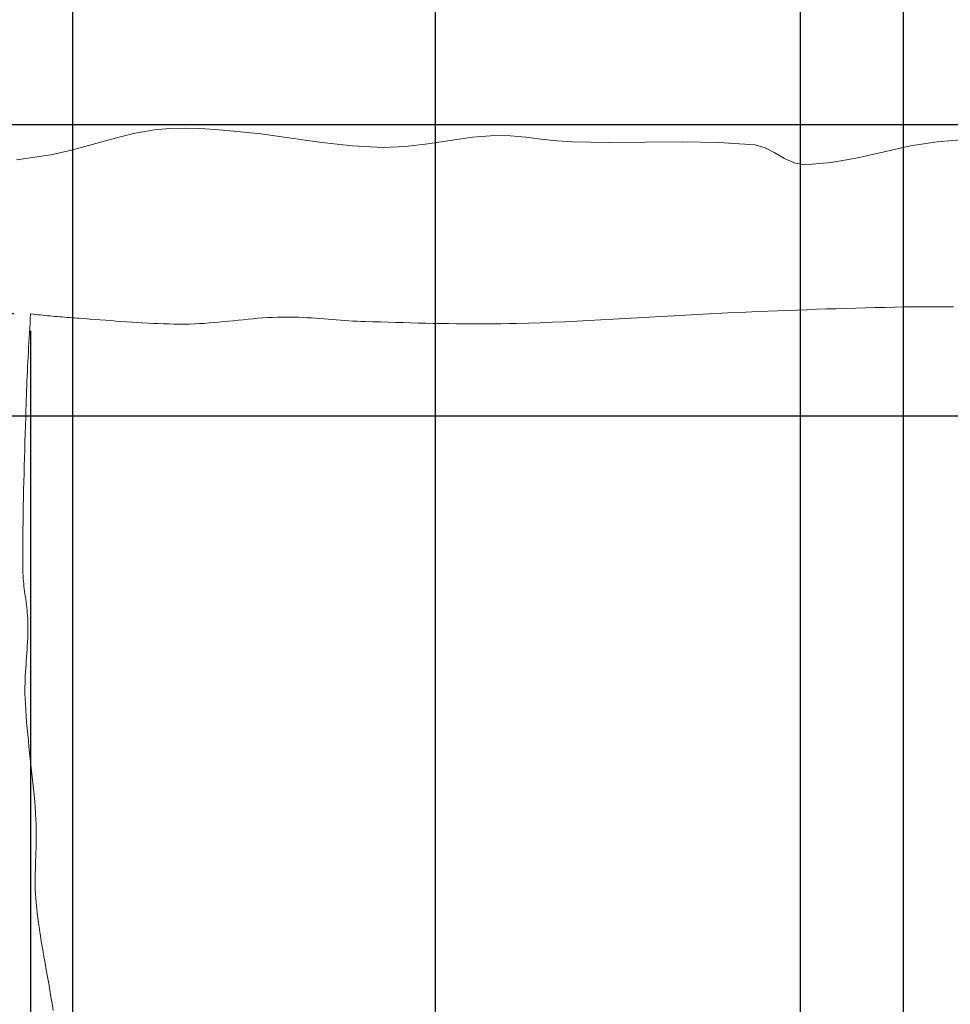
# Model space of a CAD drawing. Units: inches. Extents: x 2656 to 9931, y 1941 to 3068.
# Tile 11 of 46: x 2777 to 2811, y 2533 to 2569. Entities that reach past the tile are written whole.
import ezdxf

# ---------------------------------------------------------------- set-up
doc = ezdxf.new("R2010")
doc.units = ezdxf.units.IN
doc.layers.add('A-ANNO-DIMS', color=2, linetype='Continuous', lineweight=18)
doc.layers.add('A-FURN', color=8, linetype='Continuous', lineweight=13)
doc.styles.get("Standard").update_dxf_attribs({"font": 'arial.ttf'})
doc.dimstyles.new('ISO-25', dxfattribs={"dimtxt": 6, "dimasz": 2.5, "dimexe": 1.25, "dimexo": 0.625, "dimtad": 1, "dimdec": 0, "dimlunit": 3, "dimtxsty": 'Standard', "dimcen": 2.5, "dimadec": 0, "dimazin": 0, "dimtfac": 1, "dimtdec": 0, "dimtmove": 0, "dimatfit": 3, "dimfxl": 1, "dimarcsym": 0})

# ---------------------------------------------------------------- blocks, each defined once
blk = doc.blocks.new('BED-DOUBLE')
for p, q in [((27.981, 62.21), (27.218, 62.019)), ((28.754, 62.35), (27.981, 62.21)), ((29.308, 62.401), (28.754, 62.35)), ((29.865, 62.411), (29.308, 62.401)), ((30.423, 62.394), (29.865, 62.411)), ((30.981, 62.358), (30.423, 62.394)), ((31.538, 62.315), (30.981, 62.358)), ((32.669, 62.198), (31.538, 62.315)), ((33.797, 62.044), (32.669, 62.198)), ((40.475, 62.076), (39.653, 61.96)), ((41.299, 62.14), (40.475, 62.076)), ((41.872, 62.129), (41.299, 62.14)), ((42.443, 62.078), (41.872, 62.129)), ((43.013, 62.008), (42.443, 62.078)), ((26.459, 61.805), (25.698, 61.6)), ((27.218, 62.019), (26.459, 61.805)), ((34.924, 61.887), (33.797, 62.044)), ((36.054, 61.76), (34.924, 61.887)), ((37.187, 61.697), (36.054, 61.76)), ((38.012, 61.729), (37.187, 61.697)), ((38.833, 61.831), (38.012, 61.729)), ((39.653, 61.96), (38.833, 61.831)), ((43.584, 61.942), (43.013, 62.008)), ((44.157, 61.901), (43.584, 61.942)), ((45.504, 61.879), (44.157, 61.901)), ((46.854, 61.889), (45.504, 61.879)), ((48.203, 61.9), (46.854, 61.889)), ((49.55, 61.878), (48.203, 61.9)), ((50.893, 61.79), (49.55, 61.878)), ((51.27, 61.688), (50.893, 61.79)), ((56.625, 61.753), (55.65, 61.542)), ((57.607, 61.902), (56.625, 61.753)), ((58.764, 62.009), (57.607, 61.902)), ((24.929, 61.432), (23.668, 61.237)), ((25.698, 61.6), (24.929, 61.432)), ((51.627, 61.503), (51.27, 61.688)), ((51.978, 61.295), (51.627, 61.503)), ((55.65, 61.542), (54.677, 61.321)), ((52.336, 61.127), (51.978, 61.295)), ((52.714, 61.061), (52.336, 61.127)), ((53.7, 61.143), (52.714, 61.061)), ((54.677, 61.321), (53.7, 61.143)), ((24.187, 55.565), (24.175, 55.389)), ((24.276, 55.555), (24.187, 55.565)), ((24.366, 55.545), (24.276, 55.555)), ((24.455, 55.535), (24.366, 55.545)), ((24.544, 55.526), (24.455, 55.535)), ((24.634, 55.517), (24.544, 55.526)), ((48.773, 55.545), (48.328, 55.521)), ((49.218, 55.569), (48.773, 55.545)), ((49.663, 55.592), (49.218, 55.569)), ((50.109, 55.613), (49.663, 55.592)), ((50.554, 55.633), (50.109, 55.613)), ((50.999, 55.651), (50.554, 55.633)), ((51.36, 55.665), (50.999, 55.651)), ((51.72, 55.679), (51.36, 55.665)), ((52.081, 55.693), (51.72, 55.679)), ((52.441, 55.706), (52.081, 55.693)), ((52.802, 55.72), (52.441, 55.706)), ((53.162, 55.733), (52.802, 55.72)), ((53.522, 55.745), (53.162, 55.733)), ((53.883, 55.757), (53.522, 55.745)), ((54.244, 55.769), (53.883, 55.757)), ((54.604, 55.779), (54.244, 55.769)), ((54.965, 55.789), (54.604, 55.779)), ((55.325, 55.798), (54.965, 55.789)), ((55.686, 55.806), (55.325, 55.798)), ((56.046, 55.813), (55.686, 55.806)), ((56.407, 55.819), (56.046, 55.813)), ((56.767, 55.823), (56.407, 55.819)), ((57.128, 55.826), (56.767, 55.823)), ((57.489, 55.828), (57.128, 55.826)), ((57.849, 55.828), (57.489, 55.828)), ((58.21, 55.827), (57.849, 55.828)), ((24.164, 55.213), (24.153, 55.037)), ((24.175, 55.389), (24.164, 55.213)), ((24.723, 55.508), (24.634, 55.517)), ((24.813, 55.499), (24.723, 55.508)), ((24.902, 55.49), (24.813, 55.499)), ((24.992, 55.482), (24.902, 55.49)), ((25.081, 55.473), (24.992, 55.482)), ((25.171, 55.465), (25.081, 55.473)), ((25.26, 55.457), (25.171, 55.465)), ((25.35, 55.45), (25.26, 55.457)), ((25.439, 55.442), (25.35, 55.45)), ((25.529, 55.435), (25.439, 55.442)), ((25.619, 55.428), (25.529, 55.435)), ((25.708, 55.422), (25.619, 55.428)), ((25.798, 55.415), (25.708, 55.422)), ((25.888, 55.409), (25.798, 55.415)), ((25.977, 55.403), (25.888, 55.409)), ((26.172, 55.39), (25.977, 55.403)), ((26.366, 55.376), (26.172, 55.39)), ((26.56, 55.361), (26.366, 55.376)), ((26.754, 55.347), (26.56, 55.361)), ((26.949, 55.332), (26.754, 55.347)), ((27.143, 55.317), (26.949, 55.332)), ((27.337, 55.302), (27.143, 55.317)), ((27.531, 55.288), (27.337, 55.302)), ((27.726, 55.274), (27.531, 55.288)), ((27.92, 55.26), (27.726, 55.274)), ((28.114, 55.248), (27.92, 55.26)), ((28.309, 55.236), (28.114, 55.248)), ((28.503, 55.225), (28.309, 55.236)), ((28.698, 55.215), (28.503, 55.225)), ((28.892, 55.206), (28.698, 55.215)), ((29.087, 55.199), (28.892, 55.206)), ((29.281, 55.194), (29.087, 55.199)), ((29.476, 55.19), (29.281, 55.194)), ((29.67, 55.188), (29.476, 55.19)), ((29.865, 55.188), (29.67, 55.188)), ((30.045, 55.191), (29.865, 55.188)), ((30.226, 55.197), (30.045, 55.191)), ((30.406, 55.205), (30.226, 55.197)), ((30.586, 55.216), (30.406, 55.205)), ((30.766, 55.229), (30.586, 55.216)), ((30.946, 55.244), (30.766, 55.229)), ((31.126, 55.261), (30.946, 55.244)), ((31.306, 55.278), (31.126, 55.261)), ((31.486, 55.296), (31.306, 55.278)), ((31.665, 55.314), (31.486, 55.296)), ((31.845, 55.333), (31.665, 55.314)), ((32.025, 55.351), (31.845, 55.333)), ((32.205, 55.369), (32.025, 55.351)), ((32.385, 55.386), (32.205, 55.369)), ((32.565, 55.401), (32.385, 55.386)), ((32.745, 55.415), (32.565, 55.401)), ((32.925, 55.427), (32.745, 55.415)), ((33.105, 55.437), (32.925, 55.427)), ((33.285, 55.444), (33.105, 55.437)), ((33.466, 55.448), (33.285, 55.444)), ((33.619, 55.449), (33.466, 55.448)), ((33.772, 55.447), (33.619, 55.449)), ((33.926, 55.444), (33.772, 55.447)), ((34.079, 55.439), (33.926, 55.444)), ((34.232, 55.432), (34.079, 55.439)), ((34.385, 55.424), (34.232, 55.432)), ((34.538, 55.414), (34.385, 55.424)), ((34.691, 55.404), (34.538, 55.414)), ((34.844, 55.392), (34.691, 55.404)), ((34.997, 55.381), (34.844, 55.392)), ((35.15, 55.369), (34.997, 55.381)), ((35.303, 55.356), (35.15, 55.369)), ((35.456, 55.344), (35.303, 55.356)), ((35.609, 55.333), (35.456, 55.344)), ((35.762, 55.322), (35.609, 55.333)), ((35.915, 55.311), (35.762, 55.322)), ((36.068, 55.302), (35.915, 55.311)), ((36.221, 55.294), (36.068, 55.302)), ((36.374, 55.287), (36.221, 55.294)), ((36.528, 55.282), (36.374, 55.287)), ((36.806, 55.274), (36.528, 55.282)), ((37.084, 55.266), (36.806, 55.274)), ((37.362, 55.258), (37.084, 55.266)), ((37.641, 55.25), (37.362, 55.258)), ((37.919, 55.243), (37.641, 55.25)), ((38.198, 55.235), (37.919, 55.243)), ((38.476, 55.228), (38.198, 55.235)), ((38.754, 55.221), (38.476, 55.228)), ((39.033, 55.215), (38.754, 55.221)), ((39.311, 55.21), (39.033, 55.215)), ((39.59, 55.205), (39.311, 55.21)), ((39.868, 55.201), (39.59, 55.205)), ((40.146, 55.198), (39.868, 55.201)), ((40.425, 55.196), (40.146, 55.198)), ((40.703, 55.195), (40.425, 55.196)), ((40.982, 55.196), (40.703, 55.195)), ((41.26, 55.197), (40.982, 55.196)), ((41.538, 55.2), (41.26, 55.197)), ((41.817, 55.205), (41.538, 55.2)), ((42.095, 55.211), (41.817, 55.205)), ((42.54, 55.224), (42.095, 55.211)), ((42.986, 55.239), (42.54, 55.224)), ((43.431, 55.256), (42.986, 55.239)), ((43.877, 55.275), (43.431, 55.256)), ((44.322, 55.296), (43.877, 55.275)), ((44.767, 55.318), (44.322, 55.296)), ((45.212, 55.342), (44.767, 55.318)), ((45.657, 55.366), (45.212, 55.342)), ((46.103, 55.391), (45.657, 55.366)), ((46.548, 55.417), (46.103, 55.391)), ((46.993, 55.443), (46.548, 55.417)), ((47.438, 55.469), (46.993, 55.443)), ((47.883, 55.495), (47.438, 55.469)), ((48.328, 55.521), (47.883, 55.495)), ((24.142, 54.861), (24.132, 54.685)), ((24.153, 55.037), (24.142, 54.861)), ((24.122, 54.508), (24.112, 54.332)), ((24.132, 54.685), (24.122, 54.508)), ((24.103, 54.156), (24.093, 53.98)), ((24.112, 54.332), (24.103, 54.156)), ((24.085, 53.803), (24.076, 53.627)), ((24.093, 53.98), (24.085, 53.803)), ((24.068, 53.451), (24.06, 53.274)), ((24.076, 53.627), (24.068, 53.451)), ((24.053, 53.098), (24.046, 52.922)), ((24.06, 53.274), (24.053, 53.098)), ((24.039, 52.745), (24.033, 52.569)), ((24.046, 52.922), (24.039, 52.745)), ((24.026, 52.393), (24.021, 52.216)), ((24.033, 52.569), (24.026, 52.393)), ((24.015, 52.04), (24.006, 51.743)), ((24.021, 52.216), (24.015, 52.04)), ((24.006, 51.743), (23.997, 51.447)), ((23.997, 51.447), (23.988, 51.151)), ((23.979, 50.854), (23.97, 50.558)), ((23.988, 51.151), (23.979, 50.854)), ((23.97, 50.558), (23.961, 50.261)), ((23.961, 50.261), (23.953, 49.965)), ((23.953, 49.965), (23.944, 49.668)), ((23.937, 49.372), (23.929, 49.076)), ((23.944, 49.668), (23.937, 49.372)), ((23.929, 49.076), (23.923, 48.779)), ((23.923, 48.779), (23.917, 48.483)), ((23.917, 48.483), (23.912, 48.186)), ((23.912, 48.186), (23.907, 47.89)), ((23.904, 47.593), (23.901, 47.297)), ((23.907, 47.89), (23.904, 47.593)), ((23.901, 47.297), (23.899, 47)), ((23.899, 47), (23.899, 46.704)), ((23.899, 46.704), (23.9, 46.407)), ((23.9, 46.407), (23.902, 46.111)), ((23.902, 46.111), (23.904, 46.013)), ((23.904, 46.013), (23.908, 45.915)), ((23.908, 45.915), (23.914, 45.817)), ((23.914, 45.817), (23.922, 45.719)), ((23.922, 45.719), (23.932, 45.621)), ((23.932, 45.621), (23.942, 45.524)), ((23.942, 45.524), (23.954, 45.426)), ((23.954, 45.426), (23.966, 45.329)), ((23.966, 45.329), (23.979, 45.231)), ((23.979, 45.231), (23.992, 45.134)), ((23.992, 45.134), (24.006, 45.036)), ((24.006, 45.036), (24.019, 44.939)), ((24.019, 44.939), (24.031, 44.841)), ((24.031, 44.841), (24.043, 44.744)), ((24.043, 44.744), (24.054, 44.646)), ((24.054, 44.646), (24.064, 44.548)), ((24.064, 44.548), (24.072, 44.451)), ((24.072, 44.451), (24.079, 44.353)), ((24.079, 44.353), (24.084, 44.255)), ((24.084, 44.255), (24.087, 44.157)), ((24.087, 44.157), (24.088, 44.019)), ((24.088, 44.019), (24.087, 43.882)), ((24.078, 43.606), (24.072, 43.469)), ((24.083, 43.744), (24.078, 43.606)), ((24.087, 43.882), (24.083, 43.744)), ((24.055, 43.194), (24.046, 43.056)), ((24.064, 43.331), (24.055, 43.194)), ((24.072, 43.469), (24.064, 43.331)), ((24.036, 42.919), (24.026, 42.781)), ((24.046, 43.056), (24.036, 42.919)), ((24.007, 42.506), (23.999, 42.369)), ((24.017, 42.644), (24.007, 42.506)), ((24.026, 42.781), (24.017, 42.644)), ((23.991, 42.231), (23.985, 42.094)), ((23.999, 42.369), (23.991, 42.231)), ((23.977, 41.818), (23.976, 41.681)), ((23.98, 41.956), (23.977, 41.818)), ((23.985, 42.094), (23.98, 41.956)), ((23.976, 41.681), (23.978, 41.543)), ((23.978, 41.543), (23.982, 41.406)), ((23.982, 41.406), (23.993, 41.182)), ((23.993, 41.182), (24.006, 40.957)), ((24.006, 40.957), (24.022, 40.734)), ((24.022, 40.734), (24.04, 40.51)), ((24.04, 40.51), (24.059, 40.286)), ((24.059, 40.286), (24.08, 40.062)), ((24.08, 40.062), (24.103, 39.839)), ((24.103, 39.839), (24.126, 39.615)), ((24.126, 39.615), (24.151, 39.392)), ((24.151, 39.392), (24.175, 39.169)), ((24.175, 39.169), (24.2, 38.945)), ((24.2, 38.945), (24.225, 38.722)), ((24.225, 38.722), (24.249, 38.499)), ((24.249, 38.499), (24.272, 38.275)), ((24.272, 38.275), (24.295, 38.052)), ((24.295, 38.052), (24.316, 37.828)), ((24.316, 37.828), (24.336, 37.604)), ((24.336, 37.604), (24.354, 37.38)), ((24.354, 37.38), (24.37, 37.156)), ((24.37, 37.156), (24.383, 36.932)), ((24.383, 36.932), (24.39, 36.78)), ((24.39, 36.78), (24.394, 36.627)), ((24.394, 36.627), (24.396, 36.474)), ((24.395, 36.321), (24.394, 36.168)), ((24.396, 36.474), (24.395, 36.321)), ((24.39, 36.015), (24.386, 35.862)), ((24.394, 36.168), (24.39, 36.015)), ((24.381, 35.709), (24.376, 35.555)), ((24.386, 35.862), (24.381, 35.709)), ((24.365, 35.249), (24.361, 35.096)), ((24.37, 35.402), (24.365, 35.249)), ((24.376, 35.555), (24.37, 35.402)), ((24.358, 34.943), (24.355, 34.79)), ((24.361, 35.096), (24.358, 34.943)), ((24.355, 34.79), (24.355, 34.637)), ((24.355, 34.637), (24.356, 34.485)), ((24.356, 34.485), (24.36, 34.332)), ((24.36, 34.332), (24.367, 34.179)), ((24.367, 34.179), (24.376, 34.027)), ((24.376, 34.027), (24.389, 33.875)), ((24.389, 33.875), (24.415, 33.624)), ((24.415, 33.624), (24.444, 33.374)), ((24.444, 33.374), (24.477, 33.124)), ((24.477, 33.124), (24.512, 32.875)), ((24.512, 32.875), (24.55, 32.626)), ((24.55, 32.626), (24.59, 32.377)), ((24.59, 32.377), (24.632, 32.129)), ((24.632, 32.129), (24.675, 31.881)), ((24.675, 31.881), (24.719, 31.632)), ((24.719, 31.632), (24.763, 31.384)), ((24.763, 31.384), (24.808, 31.136)), ((24.808, 31.136), (24.852, 30.888)), ((24.852, 30.888), (24.895, 30.639)), ((24.895, 30.639), (24.937, 30.391)), ((24.937, 30.391), (24.978, 30.142)), ((24.978, 30.142), (25.017, 29.893))]:
    blk.add_line(p, q)
blk = doc.blocks.new('*D100')
at = {"layer": 'A-ANNO-DIMS', "color": 0, "lineweight": -2, "transparency": 16777216}
for p, q in [((2696.557, 2565.337), (2696.557, 2603.679)), ((2876.032, 2565.337), (2695.307, 2565.337)), ((2696.557, 2557.1), (2696.557, 2562.837)), ((2876.032, 2554.6), (2695.307, 2554.6))]:
    blk.add_line(p, q, dxfattribs=at)
at = {"layer": 'A-ANNO-DIMS', "color": 0, "transparency": 16777216}
for points in [[(2696.141, 2562.837), (2696.974, 2562.837), (2696.557, 2565.337)], [(2696.141, 2557.1), (2696.974, 2557.1), (2696.557, 2554.6)]]:
    blk.add_solid(points, dxfattribs=at)
at = {"layer": 'Defpoints', "color": 0, "transparency": 16777216}
for p in [(2696.557, 2565.337), (2876.657, 2565.337), (2876.657, 2554.6)]:
    blk.add_point(p, dxfattribs=at)
at = {"layer": 'A-ANNO-DIMS', "color": 0, "transparency": 16777216, "insert": (2692.83, 2585.758), "char_height": 6, "attachment_point": 5, "rotation": 90}
blk.add_mtext('0\'-10 1/2"', dxfattribs=at)
blk = doc.blocks.new('*D113')
at = {"layer": 'A-ANNO-DIMS', "color": 0, "lineweight": -2, "transparency": 16777216}
for p, q in [((2752.157, 2300.725), (2752.157, 2674.45)), ((2809.769, 2300.725), (2809.769, 2674.45)), ((2754.657, 2673.2), (2807.269, 2673.2))]:
    blk.add_line(p, q, dxfattribs=at)
at = {"layer": 'A-ANNO-DIMS', "color": 0, "transparency": 16777216}
for points in [[(2754.657, 2673.617), (2754.657, 2672.784), (2752.157, 2673.2)], [(2807.269, 2673.617), (2807.269, 2672.784), (2809.769, 2673.2)]]:
    blk.add_solid(points, dxfattribs=at)
at = {"layer": 'Defpoints', "color": 0, "transparency": 16777216}
for p in [(2809.769, 2673.2), (2752.157, 2300.1), (2809.769, 2300.1)]:
    blk.add_point(p, dxfattribs=at)
at = {"layer": 'A-ANNO-DIMS', "color": 0, "transparency": 16777216, "insert": (2780.963, 2676.928), "char_height": 6, "attachment_point": 5}
blk.add_mtext('4\'-9 1/2"', dxfattribs=at)
blk = doc.blocks.new('*D114')
at = {"layer": 'A-ANNO-DIMS', "color": 0, "lineweight": -2, "transparency": 16777216}
for p, q in [((2809.769, 2300.725), (2809.769, 2674.45)), ((2851.877, 2300.725), (2851.877, 2674.45)), ((2812.269, 2673.2), (2849.377, 2673.2))]:
    blk.add_line(p, q, dxfattribs=at)
at = {"layer": 'A-ANNO-DIMS', "color": 0, "transparency": 16777216}
for points in [[(2812.269, 2673.617), (2812.269, 2672.784), (2809.769, 2673.2)], [(2849.377, 2673.617), (2849.377, 2672.784), (2851.877, 2673.2)]]:
    blk.add_solid(points, dxfattribs=at)
at = {"layer": 'Defpoints', "color": 0, "transparency": 16777216}
for p in [(2851.877, 2673.2), (2809.769, 2300.1), (2851.877, 2300.1)]:
    blk.add_point(p, dxfattribs=at)
at = {"layer": 'A-ANNO-DIMS', "color": 0, "transparency": 16777216, "insert": (2830.823, 2676.891), "char_height": 6, "attachment_point": 5}
blk.add_mtext('3\'-6"', dxfattribs=at)
blk = doc.blocks.new('*D128')
at = {"layer": 'A-ANNO-DIMS', "color": 0, "lineweight": -2, "transparency": 16777216}
for p, q in [((2751.532, 2601.771), (2695.307, 2601.771)), ((2696.557, 2599.271), (2696.557, 2560.865)), ((2776.962, 2558.365), (2695.307, 2558.365))]:
    blk.add_line(p, q, dxfattribs=at)
at = {"layer": 'A-ANNO-DIMS', "color": 0, "transparency": 16777216}
for points in [[(2696.141, 2599.271), (2696.974, 2599.271), (2696.557, 2601.771)], [(2696.141, 2560.865), (2696.974, 2560.865), (2696.557, 2558.365)]]:
    blk.add_solid(points, dxfattribs=at)
at = {"layer": 'Defpoints', "color": 0, "transparency": 16777216}
for p in [(2752.157, 2601.771), (2696.557, 2558.365), (2777.587, 2558.365)]:
    blk.add_point(p, dxfattribs=at)
at = {"layer": 'A-ANNO-DIMS', "color": 0, "transparency": 16777216, "insert": (2692.828, 2580.068), "char_height": 6, "attachment_point": 5, "rotation": 90}
blk.add_mtext('3\'-7 1/2"', dxfattribs=at)
blk = doc.blocks.new('*D129')
at = {"layer": 'A-ANNO-DIMS', "color": 0, "lineweight": -2, "transparency": 16777216}
for p, q in [((2752.157, 2601.146), (2752.157, 2009.273)), ((2777.587, 2557.74), (2777.587, 2009.273)), ((2754.657, 2010.523), (2775.087, 2010.523)), ((2777.587, 2010.523), (2811.37, 2010.523))]:
    blk.add_line(p, q, dxfattribs=at)
at = {"layer": 'A-ANNO-DIMS', "color": 0, "transparency": 16777216}
for points in [[(2754.657, 2010.939), (2754.657, 2010.106), (2752.157, 2010.523)], [(2775.087, 2010.939), (2775.087, 2010.106), (2777.587, 2010.523)]]:
    blk.add_solid(points, dxfattribs=at)
at = {"layer": 'Defpoints', "color": 0, "transparency": 16777216}
for p in [(2752.157, 2601.771), (2777.587, 2558.365), (2777.587, 2010.523)]:
    blk.add_point(p, dxfattribs=at)
at = {"layer": 'A-ANNO-DIMS', "color": 0, "transparency": 16777216, "insert": (2795.728, 2014.25), "char_height": 6, "attachment_point": 5}
blk.add_mtext('2\'-1 1/2"', dxfattribs=at)
blk = doc.blocks.new('*D132')
at = {"layer": 'A-ANNO-DIMS', "color": 0, "lineweight": -2, "transparency": 16777216}
for p, q in [((2763.467, 2366.557), (2763.467, 2674.45)), ((2805.965, 2366.557), (2805.965, 2674.45)), ((2765.967, 2673.2), (2803.465, 2673.2))]:
    blk.add_line(p, q, dxfattribs=at)
at = {"layer": 'A-ANNO-DIMS', "color": 0, "transparency": 16777216}
for points in [[(2765.967, 2673.617), (2765.967, 2672.784), (2763.467, 2673.2)], [(2803.465, 2673.617), (2803.465, 2672.784), (2805.965, 2673.2)]]:
    blk.add_solid(points, dxfattribs=at)
at = {"layer": 'Defpoints', "color": 0, "transparency": 16777216}
for p in [(2805.965, 2673.2), (2763.467, 2365.932), (2805.965, 2365.932)]:
    blk.add_point(p, dxfattribs=at)
at = {"layer": 'A-ANNO-DIMS', "color": 0, "transparency": 16777216, "insert": (2784.716, 2676.93), "char_height": 6, "attachment_point": 5}
blk.add_mtext('3\'-6 1/2"', dxfattribs=at)
blk = doc.blocks.new('*D134')
at = {"layer": 'A-ANNO-DIMS', "color": 0, "lineweight": -2, "transparency": 16777216}
for p, q in [((2752.157, 2300.725), (2752.157, 2674.45)), ((2763.467, 2347.433), (2763.467, 2674.45)), ((2754.657, 2673.2), (2760.967, 2673.2)), ((2763.467, 2673.2), (2801.809, 2673.2))]:
    blk.add_line(p, q, dxfattribs=at)
at = {"layer": 'A-ANNO-DIMS', "color": 0, "transparency": 16777216}
for points in [[(2754.657, 2673.617), (2754.657, 2672.784), (2752.157, 2673.2)], [(2760.967, 2673.617), (2760.967, 2672.784), (2763.467, 2673.2)]]:
    blk.add_solid(points, dxfattribs=at)
at = {"layer": 'Defpoints', "color": 0, "transparency": 16777216}
for p in [(2763.467, 2673.2), (2763.467, 2346.808), (2752.157, 2300.1)]:
    blk.add_point(p, dxfattribs=at)
at = {"layer": 'A-ANNO-DIMS', "color": 0, "transparency": 16777216, "insert": (2783.888, 2676.928), "char_height": 6, "attachment_point": 5}
blk.add_mtext('0\'-11 1/2"', dxfattribs=at)
blk = doc.blocks.new('*D136')
at = {"layer": 'A-ANNO-DIMS', "color": 0, "lineweight": -2, "transparency": 16777216}
for p, q in [((2765.357, 2375.042), (2765.357, 2674.45)), ((2779.142, 2375.042), (2779.142, 2674.45)), ((2767.857, 2673.2), (2776.642, 2673.2)), ((2779.142, 2673.2), (2798.277, 2673.2))]:
    blk.add_line(p, q, dxfattribs=at)
at = {"layer": 'A-ANNO-DIMS', "color": 0, "transparency": 16777216}
for points in [[(2767.857, 2673.617), (2767.857, 2672.784), (2765.357, 2673.2)], [(2776.642, 2673.617), (2776.642, 2672.784), (2779.142, 2673.2)]]:
    blk.add_solid(points, dxfattribs=at)
at = {"layer": 'Defpoints', "color": 0, "transparency": 16777216}
for p in [(2779.142, 2673.2), (2765.357, 2374.417), (2779.142, 2374.417)]:
    blk.add_point(p, dxfattribs=at)
at = {"layer": 'A-ANNO-DIMS', "color": 0, "transparency": 16777216, "insert": (2789.959, 2676.838), "char_height": 6, "attachment_point": 5}
blk.add_mtext('1\'-2"', dxfattribs=at)
blk = doc.blocks.new('*D137')
at = {"layer": 'A-ANNO-DIMS', "color": 0, "lineweight": -2, "transparency": 16777216}
for p, q in [((2779.142, 2375.042), (2779.142, 2674.45)), ((2792.516, 2375.042), (2792.516, 2674.45)), ((2781.642, 2673.2), (2790.016, 2673.2)), ((2792.516, 2673.2), (2825.632, 2673.2))]:
    blk.add_line(p, q, dxfattribs=at)
at = {"layer": 'A-ANNO-DIMS', "color": 0, "transparency": 16777216}
for points in [[(2781.642, 2673.617), (2781.642, 2672.784), (2779.142, 2673.2)], [(2790.016, 2673.617), (2790.016, 2672.784), (2792.516, 2673.2)]]:
    blk.add_solid(points, dxfattribs=at)
at = {"layer": 'Defpoints', "color": 0, "transparency": 16777216}
for p in [(2792.516, 2673.2), (2779.142, 2374.417), (2792.516, 2374.417)]:
    blk.add_point(p, dxfattribs=at)
at = {"layer": 'A-ANNO-DIMS', "color": 0, "transparency": 16777216, "insert": (2810.324, 2676.928), "char_height": 6, "attachment_point": 5}
blk.add_mtext('1\'-1 1/2"', dxfattribs=at)

msp = doc.modelspace()

# ---------------------------------------------------------------- block references
at = {"layer": 'A-FURN'}
msp.add_blockref('BED-DOUBLE', (2753.4, 2502.8), dxfattribs=at)

# ---------------------------------------------------------------- dimensions: what is measured, and where the dimension line sits
at = {"layer": 'A-ANNO-DIMS'}
for base, p1, p2, picture, middle in [((2809.769, 2673.2), (2752.157, 2300.1), (2809.769, 2300.1), '*D113', (2780.963, 2676.928)), ((2763.467, 2673.2), (2752.157, 2300.1), (2763.467, 2346.808), '*D134', (2783.888, 2676.928)), ((2805.965, 2673.2), (2763.467, 2365.932), (2805.965, 2365.932), '*D132', (2784.716, 2676.93)), ((2792.516, 2673.2), (2779.142, 2374.417), (2792.516, 2374.417), '*D137', (2810.324, 2676.928)), ((2779.142, 2673.2), (2765.357, 2374.417), (2779.142, 2374.417), '*D136', (2789.959, 2676.838)), ((2851.877, 2673.2), (2809.769, 2300.1), (2851.877, 2300.1), '*D114', (2830.823, 2676.891)), ((2777.587, 2010.523), (2752.157, 2601.771), (2777.587, 2558.365), '*D129', (2795.728, 2014.25))]:
    dim = msp.add_linear_dim(base=base, p1=p1, p2=p2, dimstyle='ISO-25', override={"dimdec": 1, "dimlfac": 1, "dimrnd": 0, "dimzin": 1, "dimdsep": 46, "dimlunit": 4, "dimfrac": 2}, dxfattribs=at)
    dim.commit()
    dim.dimension.update_dxf_attribs({"geometry": picture, "text_midpoint": middle})
for base, p1, p2, picture, middle in [((2696.557, 2565.337), (2876.657, 2554.6), (2876.657, 2565.337), '*D100', (2692.83, 2585.758)), ((2696.557, 2558.365), (2752.157, 2601.771), (2777.587, 2558.365), '*D128', (2692.828, 2580.068))]:
    dim = msp.add_linear_dim(base=base, p1=p1, p2=p2, angle=90, dimstyle='ISO-25', override={"dimdec": 1, "dimlfac": 1, "dimrnd": 0, "dimzin": 1, "dimdsep": 46, "dimlunit": 4, "dimfrac": 2}, dxfattribs=at)
    dim.commit()
    dim.dimension.update_dxf_attribs({"geometry": picture, "text_midpoint": middle})

doc.saveas('drawing.dxf')
